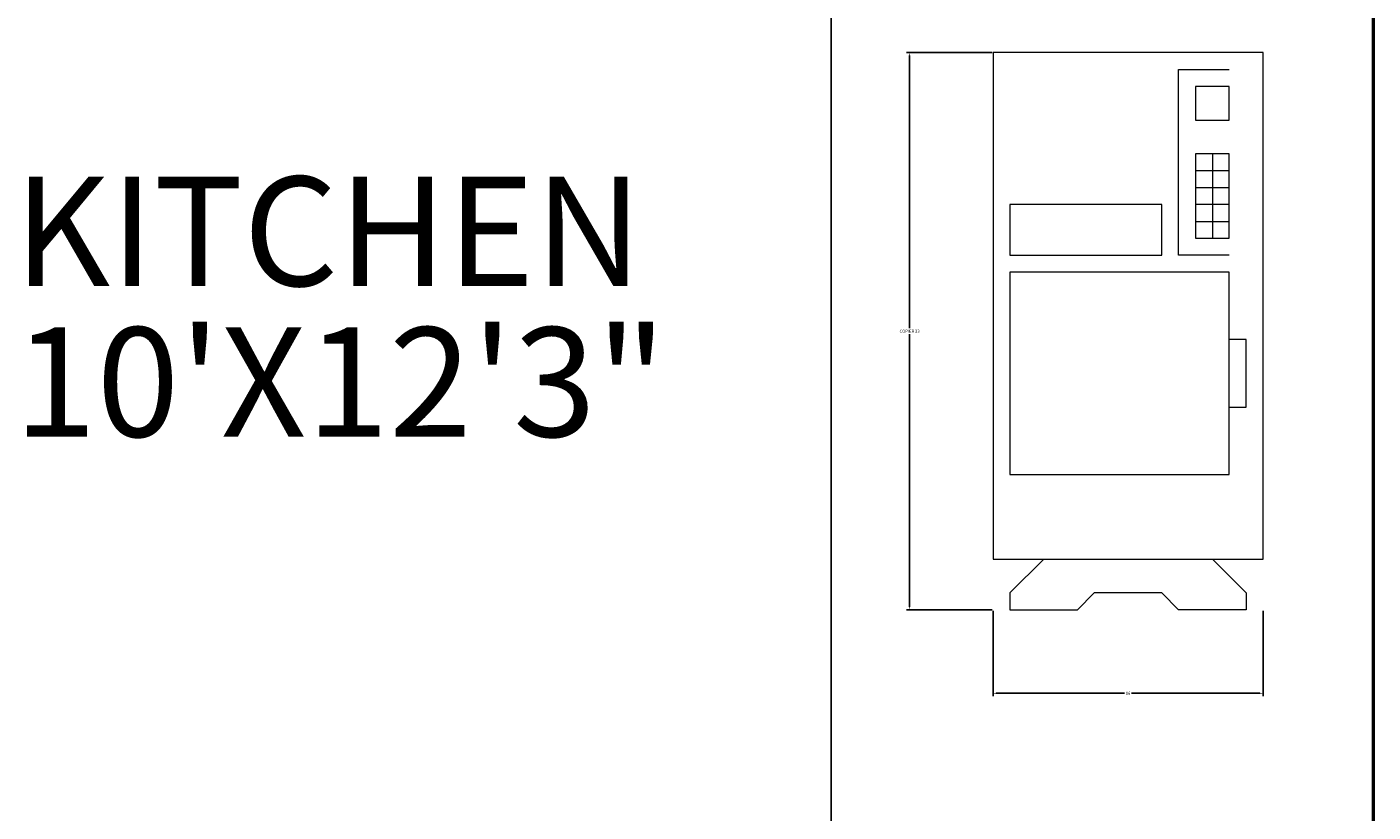
# Model space of a CAD drawing. Units: inches. Extents: x 5375 to 6084, y 16106 to 17259.
# Tile 29 of 32: x 5866 to 5946, y 16822 to 16869. Entities that reach past the tile are written whole.
import ezdxf

# ---------------------------------------------------------------- set-up
doc = ezdxf.new("R2010")
doc.units = ezdxf.units.IN
for name, color, linetype, lineweight in [('A-ANNO-DIMS', 2, 'Continuous', 18), ('A-AREA-IDEN', 5, 'Continuous', 18), ('A-EQPM', 3, 'Continuous', 18), ('A-FLOR-CASE', 3, 'Continuous', 18), ('WALL', 6, 'Continuous', 50)]:
    doc.layers.add(name, color=color, linetype=linetype, lineweight=lineweight)
doc.styles.get("Standard").update_dxf_attribs({"font": 'arial.ttf'})
doc.dimstyles.get("Standard").update_dxf_attribs({"dimtxt": 0.18, "dimasz": 0.18, "dimexe": 0.18, "dimexo": 0.0625, "dimgap": 0.09, "dimtad": 0, "dimtih": 1, "dimtoh": 1, "dimdec": 4, "dimzin": 0, "dimdsep": 46, "dimtxsty": 'Standard', "dimcen": 0.09, "dimadec": 0, "dimazin": 0, "dimtfac": 1, "dimtdec": 4, "dimtofl": 0, "dimtmove": 0, "dimatfit": 3, "dimfxl": 1, "dimtolj": 1, "dimtzin": 0, "dimarcsym": 0})

# ---------------------------------------------------------------- blocks, each defined once
blk = doc.blocks.new('Copy Machine')
for p, q in [((0, 0), (0, -16)), ((30, 0), (0, 0)), ((30, -16), (30, 0)), ((-3, -1), (-3, -5)), ((-2, -1), (-3, -1)), ((0, -3), (-2, -1)), ((5, -1), (5, -14)), ((17, -1), (5, -1)), ((17, -14), (17, -1)), ((18, -1), (18, -10)), ((21, -1), (18, -1)), ((21, -10), (21, -1)), ((-3, -5), (-2, -6)), ((-2, -10), (-2, -6)), ((-3, -11), (-2, -10)), ((18, -10), (21, -10)), ((-3, -15), (-3, -11)), ((18, -14), (18, -11)), ((18, -11), (29, -11)), ((29, -11), (29, -14)), ((24, -12), (19, -12)), ((19, -12), (19, -14)), ((20, -12), (20, -14)), ((21, -14), (21, -12)), ((22, -12), (22, -14)), ((23, -14), (23, -12)), ((24, -14), (24, -12)), ((28, -12), (26, -12)), ((26, -12), (26, -14)), ((28, -14), (28, -12)), ((0, -13), (-2, -15)), ((24, -13), (19, -13)), ((5, -14), (17, -14)), ((9, -14), (9, -15)), ((13, -15), (13, -14)), ((19, -14), (24, -14)), ((26, -14), (28, -14)), ((-2, -15), (-3, -15)), ((9, -15), (13, -15)), ((0, -16), (30, -16))]:
    blk.add_line(p, q)
blk = doc.blocks.new('*D26')
at = {"layer": 'A-ANNO-DIMS', "color": 0, "lineweight": -2, "transparency": 16777216}
for p, q in [((5923.533, 16867.209), (5918.465, 16867.209)), ((5918.645, 16867.029), (5918.645, 16850.893)), ((5918.645, 16834.389), (5918.645, 16850.526)), ((5923.533, 16834.209), (5918.465, 16834.209))]:
    blk.add_line(p, q, dxfattribs=at)
at = {"layer": 'A-ANNO-DIMS', "color": 0, "transparency": 16777216}
for points in [[(5918.615, 16867.029), (5918.675, 16867.029), (5918.645, 16867.209)], [(5918.615, 16834.389), (5918.675, 16834.389), (5918.645, 16834.209)]]:
    blk.add_solid(points, dxfattribs=at)
at = {"layer": 'Defpoints', "color": 0, "transparency": 16777216}
for p in [(5918.645, 16867.209), (5923.595, 16867.209), (5923.595, 16834.209)]:
    blk.add_point(p, dxfattribs=at)
at = {"layer": 'A-ANNO-DIMS', "color": 0, "transparency": 16777216, "insert": (5918.645, 16850.709), "char_height": 0.18, "attachment_point": 5}
blk.add_mtext('\\A1;COPIER 33', dxfattribs=at)
blk = doc.blocks.new('*D27')
at = {"layer": 'A-ANNO-DIMS', "color": 0, "lineweight": -2, "transparency": 16777216}
for p, q in [((5923.595, 16834.147), (5923.595, 16829.079)), ((5939.595, 16834.147), (5939.595, 16829.079)), ((5923.775, 16829.259), (5931.385, 16829.259)), ((5939.415, 16829.259), (5931.806, 16829.259))]:
    blk.add_line(p, q, dxfattribs=at)
at = {"layer": 'A-ANNO-DIMS', "color": 0, "transparency": 16777216}
for points in [[(5923.775, 16829.289), (5923.775, 16829.229), (5923.595, 16829.259)], [(5939.415, 16829.289), (5939.415, 16829.229), (5939.595, 16829.259)]]:
    blk.add_solid(points, dxfattribs=at)
at = {"layer": 'Defpoints', "color": 0, "transparency": 16777216}
for p in [(5923.595, 16834.209), (5939.595, 16834.209), (5923.595, 16829.259)]:
    blk.add_point(p, dxfattribs=at)
at = {"layer": 'A-ANNO-DIMS', "color": 0, "transparency": 16777216, "insert": (5931.595, 16829.259), "char_height": 0.18, "attachment_point": 5}
blk.add_mtext('\\A1;16', dxfattribs=at)
blk = doc.blocks.new('*D44')
at = {"layer": 'A-ANNO-DIMS', "color": 0, "lineweight": -2, "transparency": 16777216}
for p, q in [((5914.003, 16886.533), (5914.003, 16106.483)), ((5946.12, 16886.533), (5946.12, 16106.483)), ((5914.183, 16106.663), (5929.598, 16106.663)), ((5945.94, 16106.663), (5930.525, 16106.663))]:
    blk.add_line(p, q, dxfattribs=at)
at = {"layer": 'A-ANNO-DIMS', "color": 0, "transparency": 16777216}
for points in [[(5914.183, 16106.693), (5914.183, 16106.633), (5914.003, 16106.663)], [(5945.94, 16106.693), (5945.94, 16106.633), (5946.12, 16106.663)]]:
    blk.add_solid(points, dxfattribs=at)
at = {"layer": 'Defpoints', "color": 0, "transparency": 16777216}
for p in [(5914.003, 16886.596), (5946.12, 16886.596), (5914.003, 16106.663)]:
    blk.add_point(p, dxfattribs=at)
at = {"layer": 'A-ANNO-DIMS', "color": 0, "transparency": 16777216, "insert": (5930.062, 16106.663), "char_height": 0.18, "attachment_point": 5}
blk.add_mtext('\\A1;32.117', dxfattribs=at)

msp = doc.modelspace()

# ---------------------------------------------------------------- linework, layer by layer
at = {"layer": 'A-FLOR-CASE'}
msp.add_line((5914.0033, 16809.3651), (5914.0033, 16886.5956), dxfattribs=at)
at = {"layer": 'WALL'}
msp.add_line((5946.1199, 16891.5793), (5946.1199, 16771.5793), dxfattribs=at)

# ---------------------------------------------------------------- block references
at = {"layer": 'A-EQPM', "rotation": 90}
msp.add_blockref('Copy Machine', (5923.5952, 16837.2095), dxfattribs=at)

# ---------------------------------------------------------------- texts
at = {"layer": 'A-AREA-IDEN'}
for s, p in [('KITCHEN', (5865.5423, 16853.3866)), ('10\'X12\'3"', (5865.5423, 16844.4536))]:
    msp.add_text(s, height=6.47981, dxfattribs=at).set_placement(p)

# ---------------------------------------------------------------- dimensions: what is measured, and where the dimension line sits
at = {"layer": 'A-ANNO-DIMS'}
dim = msp.add_linear_dim(base=(5914.0033, 16106.6631), p1=(5946.1199, 16886.5956), p2=(5914.0033, 16886.5956), dimstyle='Standard', override={"dimdec": 3, "dimlfac": 1, "dimrnd": 0, "dimzin": 0, "dimdsep": 46, "dimlunit": 2}, dxfattribs=at)
dim.commit()
dim.dimension.update_dxf_attribs({"geometry": '*D44', "text_midpoint": (5930.0616, 16106.6631)})
dim = msp.add_linear_dim(base=(5918.6452, 16867.2095), p1=(5923.5952, 16834.2095), p2=(5923.5952, 16867.2095), angle=90, text='COPIER <>', dimstyle='Standard', override={"dimdec": 0, "dimlfac": 1, "dimrnd": 0, "dimzin": 0, "dimdsep": 46, "dimlunit": 2}, dxfattribs=at)
dim.commit()
dim.dimension.update_dxf_attribs({"geometry": '*D26', "text_midpoint": (5918.6452, 16850.7095)})
dim = msp.add_linear_dim(base=(5923.5952, 16829.2595), p1=(5939.5952, 16834.2095), p2=(5923.5952, 16834.2095), angle=180, dimstyle='Standard', override={"dimdec": 0, "dimlfac": 1, "dimrnd": 0, "dimzin": 0, "dimdsep": 46, "dimlunit": 2}, dxfattribs=at)
dim.commit()
dim.dimension.update_dxf_attribs({"geometry": '*D27', "text_midpoint": (5931.5952, 16829.2595)})

doc.saveas('drawing.dxf')
